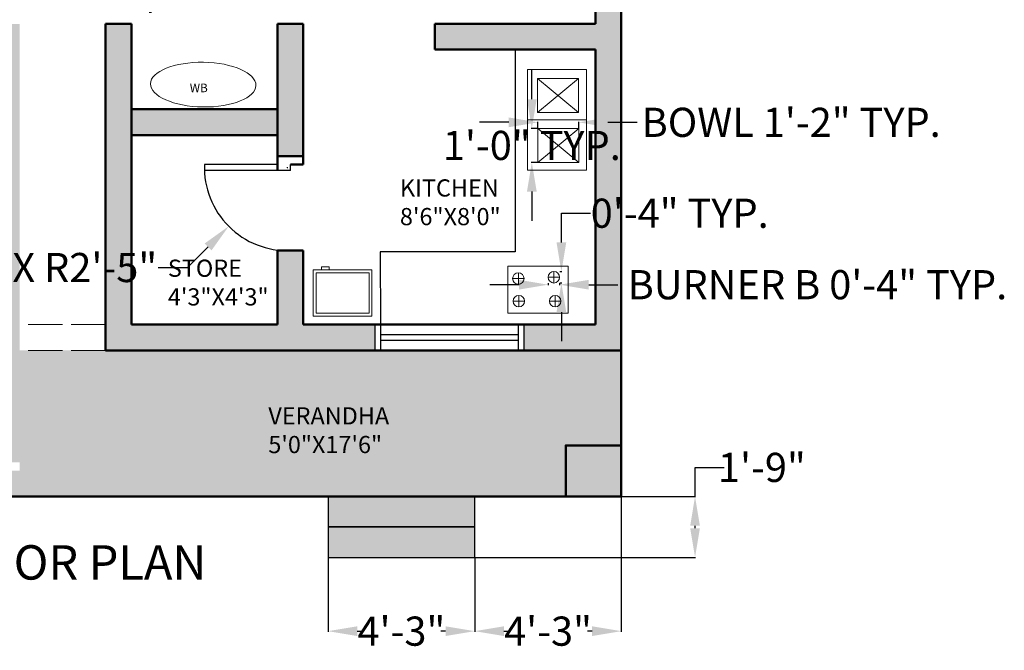
# Model space of a CAD drawing. Units: inches. Extents: x 18 to 9768, y 4 to 3529.
# Tile 5 of 6: x 9424 to 9768, y 3005 to 3225. Entities that reach past the tile are written whole.
import ezdxf

# ---------------------------------------------------------------- set-up
doc = ezdxf.new("R2010")
doc.units = ezdxf.units.IN
doc.header["$MEASUREMENT"] = 0
doc.linetypes.add('ACAD_ISO02W100', pattern=[15, 12, -3])
for name, color, linetype, lineweight in [('A-ANNO-DIMS', 2, 'Continuous', 18), ('A-ANNO-TEXT', 7, 'Continuous', 25), ('A-AREA-IDEN', 7, 'Continuous', 18), ('A-COLS', 7, 'Continuous', 50), ('A-COLS-PATT', 252, 'Continuous', 13), ('A-EQPM', 8, 'Continuous', 18), ('A-FLOR-CASE', 9, 'Continuous', 25), ('A-FLOR-FIXT', 9, 'Continuous', 18), ('A-FLOR-STRS', 7, 'Continuous', 25), ('A-WALL-OVHD', 8, 'ACAD_ISO02W100', 18), ('A-WALL-PATT', 252, 'Continuous', 13), ('WAL', 7, 'Continuous', 50)]:
    doc.layers.add(name, color=color, linetype=linetype, lineweight=lineweight)
for name, color, linetype, lineweight, true_color in [('A-DOOR', 30, 'Continuous', 25, 0xf8991e), ('A-FLOR-PATT', 254, 'Continuous', 13, 0xddb3d4), ('A-GLAZ', 177, 'Continuous', 25, 0x293189)]:
    doc.layers.add(name, color=color, linetype=linetype, lineweight=lineweight, true_color=true_color)
doc.styles.get("Standard").update_dxf_attribs({"font": 'arial.ttf'})
doc.dimstyles.get("Standard").update_dxf_attribs({"dimtxt": 10.18, "dimasz": 10.18, "dimexe": 0.18, "dimexo": 0.0625, "dimgap": 0.09, "dimtad": 0, "dimtih": 1, "dimtoh": 1, "dimdec": 0, "dimzin": 0, "dimdsep": 46, "dimlunit": 3, "dimtxsty": 'Standard', "dimcen": 0.09, "dimadec": 0, "dimazin": 0, "dimtfac": 1, "dimtdec": 0, "dimtofl": 0, "dimtmove": 0, "dimatfit": 3, "dimfxl": 1, "dimtolj": 1, "dimtzin": 0, "dimarcsym": 0})

# ---------------------------------------------------------------- blocks, each defined once
blk = doc.blocks.new('WINDOW-48')
for p, q in [((0, 0), (0, 9)), ((2, 0), (2, 9)), ((50, 0), (50, 9)), ((52, 0), (52, 9)), ((2, 5.5), (50, 5.5)), ((2, 3.5), (50, 3.5))]:
    blk.add_line(p, q)
blk = doc.blocks.new('DOOR-30-W9')
for p, q in [((25.52, 30.02), (0.02, 30.02)), ((30.02, 28.02), (0.02, 28.02)), ((30.02, 28.02), (30.02, 30.02))]:
    blk.add_line(p, q)
blk.add_arc((29.02, 29.02), 29.02, 178.0251, 271.9749)
blk = doc.blocks.new('SINK-BOWL')
for p, q in [((0, 11.84), (14.23, 0)), ((0, 0), (14.23, 11.84))]:
    blk.add_line(p, q)
blk.add_lwpolyline([(0, 11.84), (0, 11.84), (14.23, 11.84), (14.23, 11.84), (14.23, 0), (14.23, 0), (0, 0), (0, 0)], close=True)
blk = doc.blocks.new('COOKTOP-BURNER-4')
for p, q in [((1.99, 3.99), (1.99, 0)), ((0, 1.99), (3.99, 1.99))]:
    blk.add_line(p, q)
blk.add_circle((1.99, 1.99), 2)
blk = doc.blocks.new('*D39')
at = {"layer": 'A-ANNO-DIMS', "color": 0, "lineweight": -2, "transparency": 16777216}
for p, q in [((9598.76, 3132.31), (9588.58, 3132.31)), ((9608.94, 3132.84), (9608.94, 3132.13)), ((9612.93, 3132.84), (9612.93, 3132.13)), ((9623.11, 3132.31), (9633.29, 3132.31))]:
    blk.add_line(p, q, dxfattribs=at)
at = {"layer": 'A-ANNO-DIMS', "color": 0, "transparency": 16777216}
for points in [[(9598.76, 3134), (9598.76, 3130.61), (9608.94, 3132.31)], [(9623.11, 3134), (9623.11, 3130.61), (9612.93, 3132.31)]]:
    blk.add_solid(points, dxfattribs=at)
at = {"layer": 'Defpoints', "color": 0, "transparency": 16777216}
for p in [(9608.94, 3132.91), (9612.93, 3132.91), (9612.93, 3132.31)]:
    blk.add_point(p, dxfattribs=at)
at = {"layer": 'A-ANNO-DIMS', "color": 0, "transparency": 16777216, "insert": (9702.9, 3132.31), "char_height": 10.18, "attachment_point": 5}
blk.add_mtext('\\A1;BURNER B 0\'-4" TYP.', dxfattribs=at)
blk = doc.blocks.new('*D40')
at = {"layer": 'A-ANNO-DIMS', "color": 0, "lineweight": -2, "transparency": 16777216}
for p, q in [((9613.53, 3147.08), (9613.53, 3157.26)), ((9613.53, 3157.26), (9623.71, 3157.26)), ((9612.99, 3136.9), (9613.71, 3136.9)), ((9612.99, 3132.91), (9613.71, 3132.91)), ((9613.53, 3122.73), (9613.53, 3112.55))]:
    blk.add_line(p, q, dxfattribs=at)
at = {"layer": 'A-ANNO-DIMS', "color": 0, "transparency": 16777216}
for points in [[(9611.83, 3147.08), (9615.23, 3147.08), (9613.53, 3136.9)], [(9611.83, 3122.73), (9615.23, 3122.73), (9613.53, 3132.91)]]:
    blk.add_solid(points, dxfattribs=at)
at = {"layer": 'Defpoints', "color": 0, "transparency": 16777216}
for p in [(9612.93, 3136.9), (9613.53, 3136.9), (9612.93, 3132.91)]:
    blk.add_point(p, dxfattribs=at)
at = {"layer": 'A-ANNO-DIMS', "color": 0, "transparency": 16777216, "insert": (9654.83, 3157.26), "char_height": 10.18, "attachment_point": 5}
blk.add_mtext('\\A1;0\'-4" TYP.', dxfattribs=at)
blk = doc.blocks.new('*D45')
at = {"layer": 'A-ANNO-DIMS', "color": 0, "lineweight": -2, "transparency": 16777216}
for p, q in [((9595.17, 3188.98), (9584.99, 3188.98)), ((9605.35, 3186.91), (9605.35, 3189.16)), ((9619.58, 3186.91), (9619.58, 3189.16)), ((9629.76, 3188.98), (9639.94, 3188.98))]:
    blk.add_line(p, q, dxfattribs=at)
at = {"layer": 'A-ANNO-DIMS', "color": 0, "transparency": 16777216}
for points in [[(9595.17, 3190.68), (9595.17, 3187.28), (9605.35, 3188.98)], [(9629.76, 3190.68), (9629.76, 3187.28), (9619.58, 3188.98)]]:
    blk.add_solid(points, dxfattribs=at)
at = {"layer": 'Defpoints', "color": 0, "transparency": 16777216}
for p in [(9605.35, 3186.84), (9619.58, 3188.98), (9619.58, 3186.84)]:
    blk.add_point(p, dxfattribs=at)
at = {"layer": 'A-ANNO-DIMS', "color": 0, "transparency": 16777216, "insert": (9693.74, 3188.98), "char_height": 10.18, "attachment_point": 5}
blk.add_mtext('\\A1;BOWL 1\'-2" TYP.', dxfattribs=at)
blk = doc.blocks.new('*D46')
at = {"layer": 'A-ANNO-DIMS', "color": 0, "lineweight": -2, "transparency": 16777216}
for p, q in [((9603.21, 3197.02), (9603.21, 3207.2)), ((9605.29, 3186.84), (9603.03, 3186.84)), ((9605.29, 3175), (9603.03, 3175)), ((9603.21, 3164.82), (9603.21, 3154.64))]:
    blk.add_line(p, q, dxfattribs=at)
at = {"layer": 'A-ANNO-DIMS', "color": 0, "transparency": 16777216}
for points in [[(9601.52, 3197.02), (9604.91, 3197.02), (9603.21, 3186.84)], [(9601.52, 3164.82), (9604.91, 3164.82), (9603.21, 3175)]]:
    blk.add_solid(points, dxfattribs=at)
at = {"layer": 'Defpoints', "color": 0, "transparency": 16777216}
for p in [(9603.21, 3186.84), (9605.35, 3186.84), (9605.35, 3175)]:
    blk.add_point(p, dxfattribs=at)
at = {"layer": 'A-ANNO-DIMS', "color": 0, "transparency": 16777216, "insert": (9603.21, 3180.92), "char_height": 10.18, "attachment_point": 5}
blk.add_mtext('\\A1;1\'-0" TYP.', dxfattribs=at)
blk = doc.blocks.new('*D59')
at = {"layer": 'A-ANNO-DIMS', "color": 0, "lineweight": -2, "transparency": 16777216}
for p, q in [((9532.08, 3037.07), (9532.08, 3011.2)), ((9583.28, 3037.07), (9583.28, 3011.2)), ((9542.26, 3011.38), (9543.85, 3011.38)), ((9573.1, 3011.38), (9571.5, 3011.38))]:
    blk.add_line(p, q, dxfattribs=at)
at = {"layer": 'A-ANNO-DIMS', "color": 0, "transparency": 16777216}
for points in [[(9542.26, 3013.08), (9542.26, 3009.68), (9532.08, 3011.38)], [(9573.1, 3013.08), (9573.1, 3009.68), (9583.28, 3011.38)]]:
    blk.add_solid(points, dxfattribs=at)
at = {"layer": 'Defpoints', "color": 0, "transparency": 16777216}
for p in [(9532.08, 3037.13), (9583.28, 3037.13), (9583.28, 3011.38)]:
    blk.add_point(p, dxfattribs=at)
at = {"layer": 'A-ANNO-DIMS', "color": 0, "transparency": 16777216, "insert": (9557.68, 3011.38), "char_height": 10.18, "attachment_point": 5}
blk.add_mtext('\\A1;4\'-3"', dxfattribs=at)
blk = doc.blocks.new('*D60')
at = {"layer": 'A-ANNO-DIMS', "color": 0, "lineweight": -2, "transparency": 16777216}
for p, q in [((9660.18, 3058.36), (9660.18, 3068.54)), ((9660.18, 3068.54), (9670.36, 3068.54)), ((9583.35, 3058.36), (9660.36, 3058.36)), ((9660.18, 3047.31), (9660.18, 3048.18)), ((9583.35, 3037.13), (9660.36, 3037.13))]:
    blk.add_line(p, q, dxfattribs=at)
at = {"layer": 'A-ANNO-DIMS', "color": 0, "transparency": 16777216}
for points in [[(9658.49, 3048.18), (9661.88, 3048.18), (9660.18, 3058.36)], [(9658.49, 3047.31), (9661.88, 3047.31), (9660.18, 3037.13)]]:
    blk.add_solid(points, dxfattribs=at)
at = {"layer": 'Defpoints', "color": 0, "transparency": 16777216}
for p in [(9583.28, 3058.36), (9660.18, 3058.36), (9583.28, 3037.13)]:
    blk.add_point(p, dxfattribs=at)
at = {"layer": 'A-ANNO-DIMS', "color": 0, "transparency": 16777216, "insert": (9683.51, 3068.54), "char_height": 10.18, "attachment_point": 5}
blk.add_mtext('\\A1;1\'-9"', dxfattribs=at)
blk = doc.blocks.new('*D66')
at = {"layer": 'A-ANNO-DIMS', "color": 0, "lineweight": -2, "transparency": 16777216}
for p, q in [((9634.43, 3058.3), (9634.43, 3011.2)), ((9583.28, 3037.07), (9583.28, 3011.2)), ((9593.46, 3011.38), (9595.03, 3011.38)), ((9624.25, 3011.38), (9622.68, 3011.38))]:
    blk.add_line(p, q, dxfattribs=at)
at = {"layer": 'A-ANNO-DIMS', "color": 0, "transparency": 16777216}
for points in [[(9593.46, 3013.08), (9593.46, 3009.68), (9583.28, 3011.38)], [(9624.25, 3013.08), (9624.25, 3009.68), (9634.43, 3011.38)]]:
    blk.add_solid(points, dxfattribs=at)
at = {"layer": 'Defpoints', "color": 0, "transparency": 16777216}
for p in [(9634.43, 3058.36), (9583.28, 3037.13), (9634.43, 3011.38)]:
    blk.add_point(p, dxfattribs=at)
at = {"layer": 'A-ANNO-DIMS', "color": 0, "transparency": 16777216, "insert": (9608.86, 3011.38), "char_height": 10.18, "attachment_point": 5}
blk.add_mtext('\\A1;4\'-3"', dxfattribs=at)
blk = doc.blocks.new('*D82')
at = {"layer": 'A-ANNO-DIMS', "color": 0, "lineweight": -2, "transparency": 16777216}
for p, q in [((9517.84, 3173.21), (9518.02, 3173.21)), ((9517.93, 3173.12), (9517.93, 3173.3)), ((9483.02, 3138.3), (9490.22, 3145.5)), ((9472.84, 3138.3), (9483.02, 3138.3))]:
    blk.add_line(p, q, dxfattribs=at)
at = {"layer": 'A-ANNO-DIMS', "color": 0, "transparency": 16777216}
blk.add_solid([(9489.02, 3146.7), (9491.42, 3144.3), (9497.42, 3152.7)], dxfattribs=at)
at = {"layer": 'Defpoints', "color": 0, "transparency": 16777216}
for p in [(9517.93, 3173.21), (9497.42, 3152.7)]:
    blk.add_point(p, dxfattribs=at)
at = {"layer": 'A-ANNO-DIMS', "color": 0, "transparency": 16777216, "insert": (9443.32, 3138.3), "char_height": 10.18, "attachment_point": 5}
blk.add_mtext('\\A1;2X R2\'-5"', dxfattribs=at)
blk = doc.blocks.new('*D84')
at = {"layer": 'A-ANNO-DIMS', "color": 0, "lineweight": -2, "transparency": 16777216}
for p, q in [((9499.78, 3262.71), (9499.96, 3262.71)), ((9499.87, 3262.62), (9499.87, 3262.8)), ((9499.49, 3234.76), (9499.63, 3244.93)), ((9489.31, 3234.76), (9499.49, 3234.76))]:
    blk.add_line(p, q, dxfattribs=at)
at = {"layer": 'A-ANNO-DIMS', "color": 0, "transparency": 16777216}
blk.add_solid([(9497.93, 3244.96), (9501.32, 3244.91), (9499.77, 3255.11)], dxfattribs=at)
at = {"layer": 'Defpoints', "color": 0, "transparency": 16777216}
for p in [(9499.87, 3262.71), (9499.77, 3255.11)]:
    blk.add_point(p, dxfattribs=at)
at = {"layer": 'A-ANNO-DIMS', "color": 0, "transparency": 16777216, "insert": (9448.02, 3234.76), "char_height": 10.18, "attachment_point": 5}
blk.add_mtext('\\A1;5X R0\'-7 1/2"', dxfattribs=at)

msp = doc.modelspace()

# ---------------------------------------------------------------- hatches: boundary and pattern name
at = {"layer": 'A-COLS-PATT'}
h = msp.add_hatch(color=256, dxfattribs=at)
h.dxf.hatch_style = 1
h.paths.add_polyline_path([(9634.43, 3076.24), (9615.06, 3076.24), (9615.06, 3058.36), (9634.43, 3058.36)])
at = {"layer": 'A-FLOR-PATT'}
h = msp.add_hatch(color=256, dxfattribs=at)
h.dxf.hatch_style = 1
h.paths.add_polyline_path([(9583.28, 3058.36), (9532.08, 3058.36), (9532.08, 3047.74), (9583.28, 3047.74)])
h.paths.add_polyline_path([(9583.28, 3047.74), (9532.08, 3047.74), (9532.08, 3037.13), (9583.28, 3037.13)])
h.paths.add_polyline_path([(9615.06, 3076.24), (9634.43, 3076.24), (9634.43, 3109.36), (9625.43, 3109.36), (9454.43, 3109.36), (9424.43, 3109.36), (9424.43, 3106.36), (9417.93, 3106.36, 0.397579), (9383.93, 3072.36), (9419.93, 3072.36), (9419.93, 3070.36), (9424.43, 3070.36), (9424.43, 3067.36), (9424.43, 3058.36), (9615.06, 3058.36)])
h.paths.add_polyline_path([(9509.39, 3070.22), (9559.29, 3070.22), (9559.29, 3092.61), (9509.39, 3092.61)], flags=24)
at = {"layer": 'A-WALL-PATT'}
h = msp.add_hatch(color=256, dxfattribs=at)
h.dxf.hatch_style = 1
h.paths.add_polyline_path([(9424.43, 3490.36), (9363.42, 3490.36), (9363.42, 3481.36), (9373.43, 3481.36), (9382.43, 3481.36), (9415.43, 3481.36), (9415.43, 3373.36), (9415.43, 3364.36), (9424.43, 3364.36), (9424.43, 3373.36), (9424.43, 3481.36)])
h.paths.add_polyline_path([(9527.43, 3490.36), (9472.43, 3490.36), (9472.43, 3481.36), (9472.43, 3373.36), (9472.43, 3364.36), (9481.43, 3364.36), (9481.43, 3373.36), (9481.43, 3481.36), (9527.43, 3481.36)])
h.paths.add_polyline_path([(9311.42, 3490.36), (9250.43, 3490.36), (9250.43, 3353.86), (9259.43, 3353.86), (9259.43, 3364.36), (9301.43, 3364.36), (9301.43, 3315.36), (9301.43, 3306.36), (9310.43, 3306.36), (9310.43, 3315.36), (9310.43, 3364.36), (9382.43, 3364.36), (9382.43, 3368.86, -0.017236), (9382.43, 3370.86), (9382.43, 3373.36), (9259.43, 3373.36), (9259.43, 3481.36), (9311.42, 3481.36)])
h.paths.add_polyline_path([(9376.43, 3216.86, -0.014283), (9376.43, 3218.86), (9376.43, 3223.36), (9259.43, 3223.36), (9259.43, 3238.86), (9250.43, 3238.86), (9250.43, 3058.36), (9311.43, 3058.36), (9311.43, 3067.36), (9259.43, 3067.36), (9259.43, 3214.36), (9376.43, 3214.36)])
h.paths.add_polyline_path([(9382.43, 3364.36), (9373.43, 3364.36), (9373.43, 3315.36), (9347, 3315.36), (9347, 3306.36), (9382.43, 3306.36)], flags=0)
h.paths.add_polyline_path([(9277.41, 3315.36), (9259.43, 3315.36), (9259.43, 3325.86), (9250.43, 3325.86), (9250.43, 3290.86), (9259.43, 3290.86), (9259.43, 3306.36), (9277.41, 3306.36)])
h.paths.add_polyline_path([(9424.43, 3214.36), (9424.43, 3223.36), (9415.43, 3223.36), (9415.43, 3214.36), (9415.43, 3106.36), (9417.93, 3106.36, -0.014283), (9419.93, 3106.36), (9424.43, 3106.36), (9424.43, 3109.36), (9424.43, 3118.36)])
h.paths.add_polyline_path([(9463.43, 3214.36), (9463.43, 3223.36), (9454.43, 3223.36), (9454.43, 3214.36), (9454.43, 3118.36), (9454.43, 3109.36), (9548.43, 3109.36), (9548.43, 3118.36), (9523.43, 3118.36), (9523.43, 3144.21), (9518.93, 3144.21, -0.017236), (9516.93, 3144.21), (9514.43, 3144.21), (9514.43, 3118.36), (9463.43, 3118.36)])
h.paths.add_polyline_path([(9523.43, 3214.36), (9523.43, 3223.36), (9514.43, 3223.36), (9514.43, 3214.36), (9514.43, 3177.21), (9523.43, 3177.21)], flags=17)
h.paths.add_polyline_path([(9514.43, 3193.54), (9463.43, 3193.54), (9463.43, 3184.54), (9514.43, 3184.54)], flags=17)
h.paths.add_polyline_path([(9634.43, 3267.86), (9625.43, 3267.86), (9625.43, 3223.36), (9569.35, 3223.36), (9569.35, 3214.36), (9625.43, 3214.36), (9625.43, 3118.36), (9600.43, 3118.36), (9600.43, 3109.36), (9625.43, 3109.36), (9634.43, 3109.36)])
h.paths.add_polyline_path([(9634.43, 3490.36), (9579.43, 3490.36), (9579.43, 3481.36), (9625.43, 3481.36), (9625.43, 3373.36), (9520.43, 3373.36), (9520.43, 3370.86, -0.014283), (9520.43, 3368.86), (9520.43, 3364.36), (9625.43, 3364.36), (9625.43, 3319.86), (9634.43, 3319.86)])
h.paths.add_polyline_path([(9424.43, 3067.36), (9415.43, 3067.36), (9363.43, 3067.36), (9363.43, 3058.36), (9424.43, 3058.36)])

# ---------------------------------------------------------------- linework, layer by layer
at = {"layer": 'A-COLS'}
msp.add_lwpolyline([(9634.43, 3058.36), (9634.43, 3058.36), (9615.06, 3058.36), (9615.06, 3058.36), (9615.06, 3076.24), (9615.06, 3076.24), (9634.43, 3076.24), (9634.43, 3076.24)], close=True, dxfattribs=at)
at = {"layer": 'A-EQPM'}
for points in [[(9529.78, 3137.48), (9529.78, 3137.48), (9532.52, 3137.48), (9532.52, 3137.48), (9532.52, 3138.55), (9532.52, 3138.55), (9529.78, 3138.55), (9529.78, 3138.55)], [(9594.8, 3138.8), (9594.8, 3138.8), (9615.94, 3138.8), (9615.94, 3138.8), (9615.94, 3122.37), (9615.94, 3122.37), (9594.8, 3122.37), (9594.8, 3122.37)], [(9526.95, 3137.48), (9526.95, 3137.48), (9547.39, 3137.48), (9547.39, 3137.48), (9547.39, 3121.35), (9547.39, 3121.35), (9526.95, 3121.35), (9526.95, 3121.35)], [(9527.95, 3136.48), (9546.39, 3136.48), (9546.39, 3122.35), (9527.95, 3122.35)]]:
    msp.add_lwpolyline(points, close=True, dxfattribs=at)
at = {"layer": 'A-FLOR-CASE'}
for p, q in [((9597.39, 3214.36), (9597.39, 3143.73)), ((9597.39, 3143.73), (9550.28, 3143.73)), ((9550.28, 3143.73), (9550.43, 3118.36))]:
    msp.add_line(p, q, dxfattribs=at)
at = {"layer": 'A-FLOR-FIXT'}
msp.add_line((9622.29, 3189.86), (9601.66, 3189.86), dxfattribs=at)
msp.add_lwpolyline([(9601.66, 3207.39), (9601.66, 3207.39), (9622.29, 3207.39), (9622.29, 3207.39), (9622.29, 3172.34), (9622.29, 3172.34), (9601.66, 3172.34), (9601.66, 3172.34)], close=True, dxfattribs=at)
msp.add_ellipse((9488.51, 3202.15), major_axis=(18.4, -0.29), ratio=0.424123, dxfattribs=at)
at = {"layer": 'A-FLOR-STRS'}
for points in [[(9583.28, 3058.36), (9583.28, 3058.36), (9532.08, 3058.36), (9532.08, 3058.36), (9532.08, 3047.74), (9532.08, 3047.74), (9583.28, 3047.74), (9583.28, 3047.74)], [(9583.28, 3047.74), (9583.28, 3047.74), (9532.08, 3047.74), (9532.08, 3047.74), (9532.08, 3037.13), (9532.08, 3037.13), (9583.28, 3037.13), (9583.28, 3037.13)]]:
    msp.add_lwpolyline(points, close=True, dxfattribs=at)
at = {"layer": 'A-WALL-OVHD'}
for p, q in [((9454.43, 3118.36), (9424.43, 3118.36)), ((9454.43, 3109.36), (9424.43, 3109.36))]:
    msp.add_line(p, q, dxfattribs=at)
at = {"layer": 'WAL'}
for p, q in [((9634.43, 3490.36), (9634.43, 3058.36)), ((9625.43, 3364.36), (9625.43, 3223.36)), ((9463.43, 3223.36), (9454.43, 3223.36)), ((9454.43, 3214.36), (9454.43, 3223.36)), ((9463.43, 3214.36), (9463.43, 3223.36)), ((9523.43, 3223.36), (9514.43, 3223.36)), ((9514.43, 3214.36), (9514.43, 3223.36)), ((9523.43, 3214.36), (9523.43, 3223.36)), ((9625.43, 3223.36), (9569.35, 3223.36)), ((9569.35, 3223.36), (9569.35, 3214.36)), ((9454.43, 3214.36), (9454.43, 3118.36)), ((9463.43, 3214.36), (9463.43, 3118.36)), ((9514.43, 3214.36), (9514.43, 3172.21)), ((9523.43, 3214.36), (9523.43, 3174.21)), ((9625.43, 3214.36), (9569.35, 3214.36)), ((9625.43, 3214.36), (9625.43, 3118.36)), ((9463.43, 3193.54), (9514.43, 3193.54)), ((9463.43, 3184.54), (9514.43, 3184.54)), ((9523.43, 3177.21), (9514.43, 3177.21)), ((9523.43, 3174.21), (9518.93, 3174.21)), ((9514.43, 3144.41), (9514.43, 3118.36)), ((9523.43, 3144.21), (9514.43, 3144.21)), ((9523.43, 3144.21), (9523.43, 3118.36)), ((9454.43, 3118.36), (9454.43, 3109.36)), ((9514.43, 3118.36), (9463.43, 3118.36)), ((9625.43, 3118.36), (9523.43, 3118.36)), ((9625.43, 3109.36), (9454.43, 3109.36)), ((9625.43, 3109.36), (9634.43, 3109.36)), ((9634.43, 3058.36), (9250.43, 3058.36))]:
    msp.add_line(p, q, dxfattribs=at)

# ---------------------------------------------------------------- block references
at = {"layer": 'A-DOOR'}
msp.add_blockref('DOOR-30-W9', (9488.92, 3144.2), dxfattribs=at)
at = {"layer": 'A-EQPM'}
for p, rotation in [((9600.5, 3132.46), 90), ((9600.67, 3124.59), 89.99999999998694), ((9613.34, 3124.59), 89.99999999998694)]:
    msp.add_blockref('COOKTOP-BURNER-4', p, dxfattribs=dict(at, rotation=rotation))
msp.add_blockref('COOKTOP-BURNER-4', (9608.94, 3132.91), dxfattribs=at)
at = {"layer": 'A-FLOR-FIXT'}
for p in [(9605.22, 3192.47), (9605.35, 3175)]:
    msp.add_blockref('SINK-BOWL', p, dxfattribs=at)
at = {"layer": 'A-GLAZ', "rotation": 180}
msp.add_blockref('WINDOW-48', (9600.43, 3118.36), dxfattribs=at)

# ---------------------------------------------------------------- texts
at = {"layer": 'A-ANNO-TEXT', "attachment_point": 1}
for s, width, insert, char_height in [('WB', 9.8121, (9483.82, 3202.5), 3), ('GROUND FLOOR PLAN', 445.7923, (9319.88, 3041.38), 12)]:
    msp.add_mtext_dynamic_manual_height_columns(s, width=width, gutter_width=1, heights=[0], dxfattribs=dict(at, insert=insert, char_height=char_height))
at = {"layer": 'A-AREA-IDEN', "char_height": 6, "attachment_point": 1}
for s, insert in [('KITCHEN\\P8\'6"X8\'0"', (9557.17, 3169.08)), ('STORE\\P4\'3"X4\'3"', (9476.17, 3141.06)), ('VERANDHA\\P5\'0"X17\'6"', (9511.24, 3089.52))]:
    msp.add_mtext_dynamic_manual_height_columns(s, width=61.6465, gutter_width=1, heights=[0], dxfattribs=dict(at, insert=insert))

# ---------------------------------------------------------------- dimensions: what is measured, and where the dimension line sits
at = {"layer": 'A-ANNO-DIMS'}
for center, mpoint, text, picture, middle in [((9499.87, 3262.71), (9499.77, 3255.11), '5X <>', '*D84', (9448.02, 3234.76)), ((9517.93, 3173.21), (9497.42, 3152.7), '2X <>', '*D82', (9443.32, 3138.3))]:
    dim = msp.add_radius_dim(center=center, mpoint=mpoint, text=text, dimstyle='Standard', override={"dimdec": 1, "dimlfac": 1, "dimrnd": 0, "dimzin": 1, "dimdsep": 46, "dimlunit": 4, "dimfrac": 2}, dxfattribs=at)
    dim.commit()
    dim.dimension.update_dxf_attribs({"geometry": picture, "text_midpoint": middle})
for base, p1, p2, text, picture, middle in [((9619.58, 3188.98), (9605.35, 3186.84), (9619.58, 3186.84), 'BOWL <> TYP.', '*D45', (9693.74, 3188.98)), ((9612.93, 3132.31), (9608.94, 3132.91), (9612.93, 3132.91), 'BURNER B <> TYP.', '*D39', (9702.9, 3132.31))]:
    dim = msp.add_linear_dim(base=base, p1=p1, p2=p2, text=text, dimstyle='Standard', override={"dimdec": 1, "dimlfac": 1, "dimrnd": 0, "dimzin": 1, "dimdsep": 46, "dimlunit": 4, "dimfrac": 2}, dxfattribs=at)
    dim.commit()
    dim.dimension.update_dxf_attribs({"geometry": picture, "text_midpoint": middle})
for base, p1, p2, picture, middle in [((9603.21, 3186.84), (9605.35, 3175), (9605.35, 3186.84), '*D46', (9603.21, 3180.92)), ((9613.53, 3136.9), (9612.93, 3132.91), (9612.93, 3136.9), '*D40', (9654.83, 3157.26))]:
    dim = msp.add_linear_dim(base=base, p1=p1, p2=p2, angle=90, text='<> TYP.', dimstyle='Standard', override={"dimdec": 1, "dimlfac": 1, "dimrnd": 0, "dimzin": 1, "dimdsep": 46, "dimlunit": 4, "dimfrac": 2}, dxfattribs=at)
    dim.commit()
    dim.dimension.update_dxf_attribs({"geometry": picture, "text_midpoint": middle})
dim = msp.add_linear_dim(base=(9660.18, 3058.36), p1=(9583.28, 3037.13), p2=(9583.28, 3058.36), angle=90, dimstyle='Standard', override={"dimdec": 1, "dimlfac": 1, "dimrnd": 0, "dimzin": 1, "dimdsep": 46, "dimlunit": 4, "dimfrac": 2}, dxfattribs=at)
dim.commit()
dim.dimension.update_dxf_attribs({"geometry": '*D60', "text_midpoint": (9683.51, 3068.54)})
for base, p1, p2, picture, middle in [((9634.4338, 3011.3784), (9583.284, 3037.1284), (9634.4338, 3058.3604), '*D66', (9608.8589, 3011.3784)), ((9583.28, 3011.38), (9532.08, 3037.13), (9583.28, 3037.13), '*D59', (9557.68, 3011.38))]:
    dim = msp.add_linear_dim(base=base, p1=p1, p2=p2, dimstyle='Standard', override={"dimdec": 1, "dimlfac": 1, "dimrnd": 0, "dimzin": 1, "dimdsep": 46, "dimlunit": 4, "dimfrac": 2}, dxfattribs=at)
    dim.commit()
    dim.dimension.update_dxf_attribs({"geometry": picture, "text_midpoint": middle})

doc.saveas('drawing.dxf')
